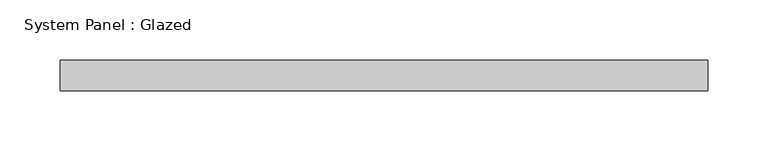
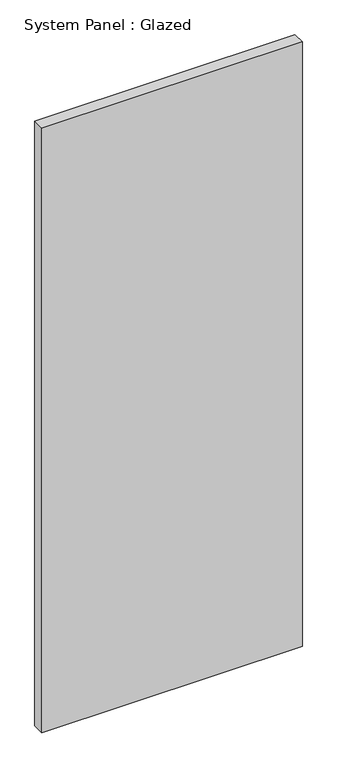
"""IFC4 building model written with IfcOpenShell, lengths in millimetres: plate geometry, System Panel : Glazed."""

from ifc_helpers import new_model, si_unit, origin, origin_with_axes, place, context, project, spatial, polyline, outline, extrude, source, transform, mapped, element, save


def system_panel_glazed_63ee4140(model_context):
    return source(origin(), model_context, "Body", "SweptSolid", [
        extrude(outline(polyline([(269.875, 19.05), (-269.875, 19.05), (-269.875, 44.45), (269.875, 44.45), (269.875, 19.05)])), origin_with_axes(), (0.0, 0.0, 1.0), 1324.8907014),
    ])


if __name__ == "__main__":
    model = new_model("IFC4")
    model_context = context("Model", 3, world=origin())
    ifc_project = project(units=[si_unit("LENGTHUNIT", "METRE", prefix="MILLI")], contexts=[model_context])
    site = spatial("IfcSite", under=ifc_project)
    building = spatial("IfcBuilding", under=site)
    placement = place(None, origin())
    system_panel_glazed_shape = system_panel_glazed_63ee4140(model_context)
    element("IfcPlate", 1, ObjectType="System Panel : Glazed", at=placement, inside=building, context=model_context, shape_type="MappedRepresentation", body=[
        mapped(system_panel_glazed_shape, transform((0.0, 0.0, 0.0), x_axis=(1.0, 0.0, 0.0), y_axis=(0.0, 1.0, 0.0), z_axis=(0.0, 0.0, 1.0))),
    ])
    save(model, "model.ifc")

# Revit data of these elements
# Type "System Panel : Glazed"
#   Construction Type Id = "GSP4R"
#   Analytic Construction = "1/8 in Pilkington single glazing"
#   Visual Light Transmittance = 0.9
#   Solar Heat Gain Coefficient = 0.86
#   Heat Transfer Coefficient (U) = 1.18115 BTU/(h·ft²·°F)
#   Define Thermal Properties by = 1
# Element 1 (IfcPlate, "System Panel : Glazed")
#   Materials on its faces: "Glass"
# Materials
#   "Glass": class "Glass", colour RGB 0 128 192, transparency 0.75, Description = "Soda Lime Glass", Cost = 0
